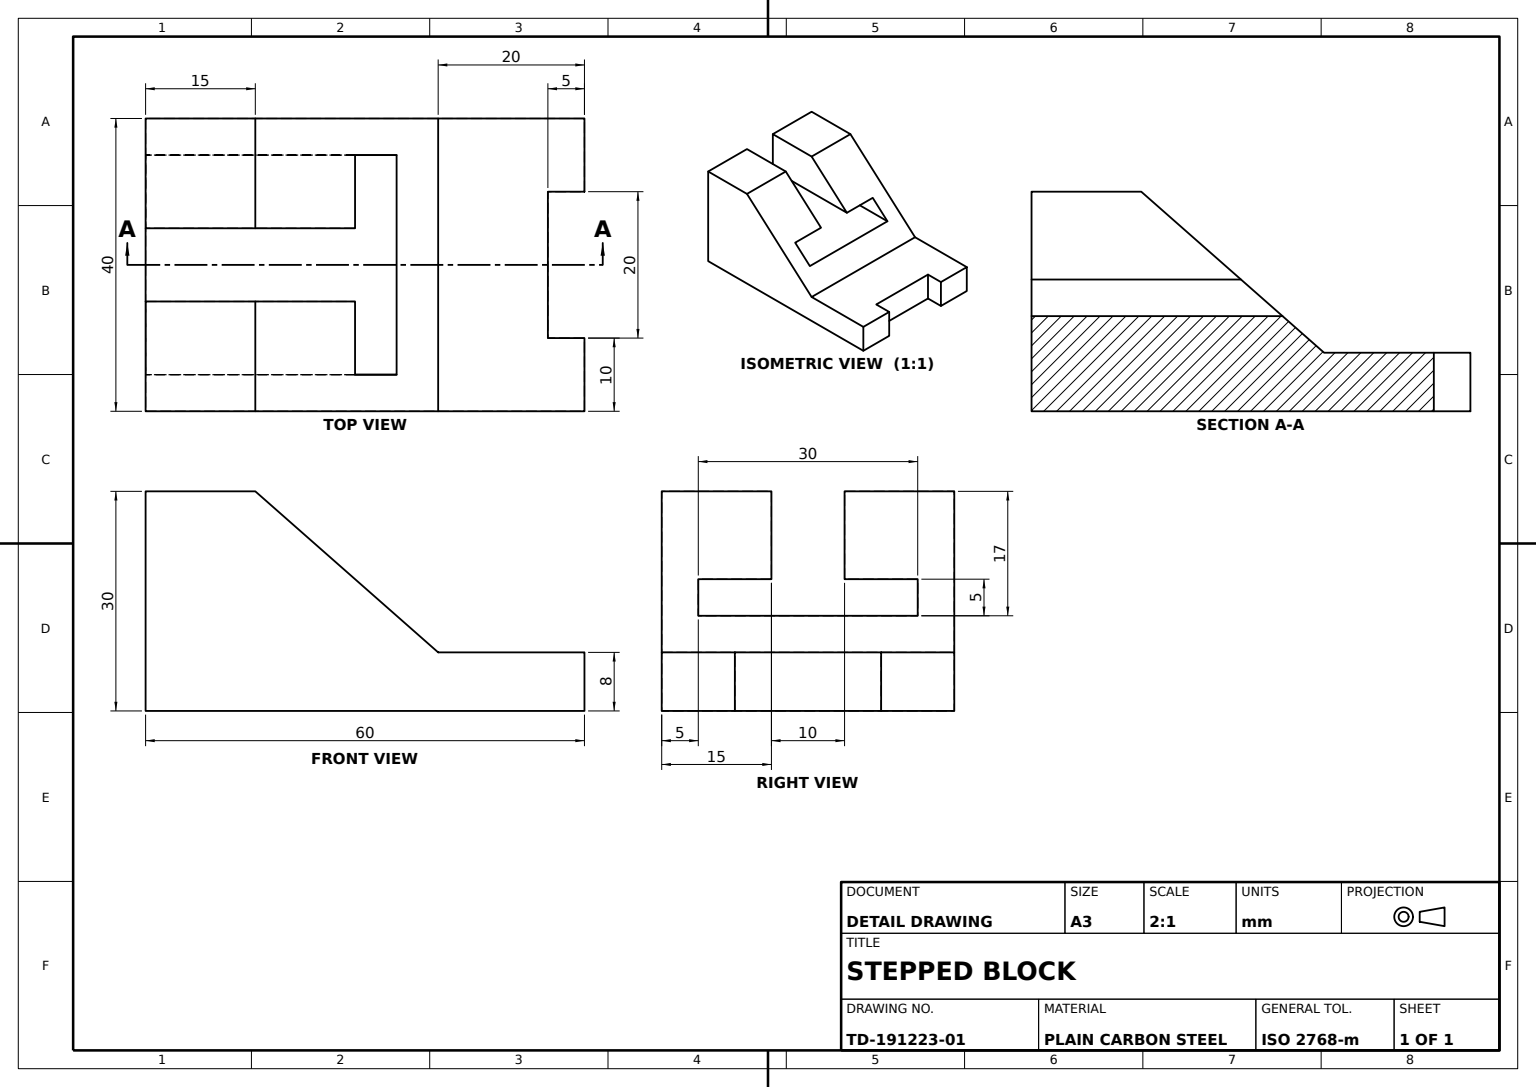
SolidWorks part; units mm, degrees
material "Plain Carbon Steel"
ref_plane "Front Plane" through (0, 0, 0) normal (0, 0, 1) x (1, 0, 0)
ref_plane "Top Plane" through (0, 0, 0) normal (0, 1, 0) x (1, 0, 0)
ref_plane "Right Plane" through (0, 0, 0) normal (1, 0, 0) x (0, 0, -1)
sketch "Base Plate Sketch" plane through (0, 0, 0) normal (0, 1, 0) x (1, 0, 0)
  line L0 (0, 0) -> (20, 0)
  line L1 (20, 0) -> (20, 60)
  line L2 (20, 60) -> (-20, 60)
  line L3 (-20, 60) -> (-20, 0)
  line L4 (-20, 0) -> (0, 0)
  dimension "D1" = 20
  dimension "D2" = 60
extrude "Base Plate 8mm" add sketch "Base Plate Sketch" along normal blind 8
sketch "Upright Lower Sketch" plane through (20, 0, 0) normal (1, 0, 0) x (0, 0, -1)
  line L0 (60, 8) -> (60, 30)
  line L1 (60, 30) -> (45, 30)
  line L2 (60, 8) -> (20, 8)
  line L3 (0, 8) -> (60, 8) construction
  line L4 (20, 8) -> (45, 30)
  line L5 (0, 0) -> (60, 0) construction
  dimension "D1" = 15
  dimension "D2" = 40
  dimension "D3" = 30
extrude "Upright Lower 15mm" add sketch "Upright Lower Sketch" against normal blind 15
sketch "Upright Middle Sketch" plane through (-20, 0, 0) normal (-1, 0, 0) x (0, 0, 1)
  line L0 (-60, 8) -> (-60, 30)
  line L1 (-60, 30) -> (-45, 30)
  line L2 (-45, 30) -> (-20, 8)
  line L3 (-20, 8) -> (-60, 8)
extrude "Upright Middle 15mm" add sketch "Upright Middle Sketch" against normal blind 15
sketch "Upright Top Sketch" plane through (0, 8, 0) normal (0, 1, 0) x (1, 0, 0)
  line L0 (-5, 60) -> (5, 60)
  line L1 (5, 60) -> (5, 20)
  line L2 (5, 20) -> (-5, 20)
  line L3 (-5, 20) -> (-5, 60)
extrude "Upright Top 10mm" add sketch "Upright Top Sketch" along normal blind 10
sketch "Slope Cut Sketch" plane through (5, 0, 0) normal (1, 0, 0) x (0, 0, -1)
  line L0 (20, 8) -> (20, 18)
  line L1 (20, 18) -> (31.3636, 18)
  line L2 (31.3636, 18) -> (20, 8)
extrude "Slope Cut" cut sketch "Slope Cut Sketch" against normal blind 40
sketch "Centre Slot Sketch" plane through (0, 0, -60) normal (0, 0, -1) x (-1, 0, 0)
  line L0 (-20, 30) -> (-20, 0) construction
  line L1 (-5, 30) -> (-20, 30) construction
  line L2 (0, 13) -> (15, 13)
  line L3 (15, 13) -> (15, 18)
  line L4 (15, 18) -> (-15, 18)
  line L5 (-15, 18) -> (-15, 13)
  line L6 (-15, 13) -> (0, 13)
  dimension "D1" = 5
  dimension "D2" = 20
  dimension "D3" = 17
extrude "Centre Slot Cut" cut sketch "Centre Slot Sketch" against normal blind 40
sketch "Front Notch Sketch" plane through (0, 8, 0) normal (0, 1, 0) x (1, 0, 0)
  line L0 (-20, 20) -> (-20, 0) construction
  line L1 (0, 5) -> (10, 5)
  line L2 (10, 5) -> (10, 0)
  line L3 (-20, 0) -> (20, 0) construction
  line L4 (10, 0) -> (-10, 0)
  line L5 (-10, 0) -> (-10, 5)
  line L6 (-10, 5) -> (0, 5)
  line L7 (-20, 20) -> (20, 20) construction
  dimension "D1" = 10
  dimension "D2" = 20
  dimension "D3" = 15
extrude "Front Notch Cut" cut sketch "Front Notch Sketch" against normal blind 40
